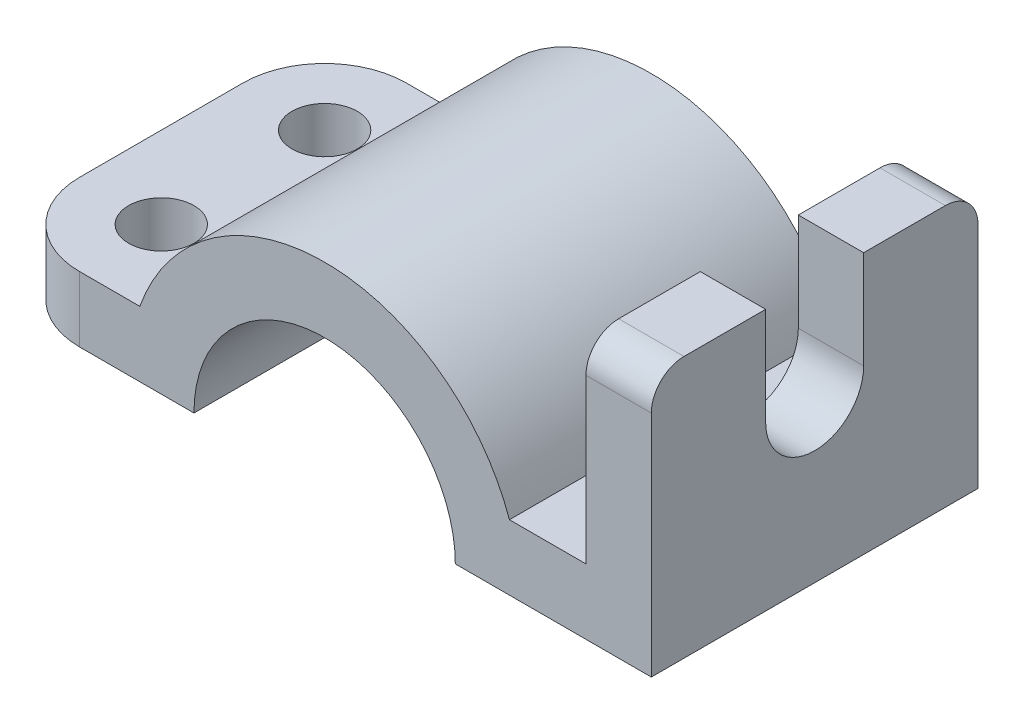
ISO-10303-21;
HEADER;
FILE_DESCRIPTION(('STEP AP214'),'2;1');
FILE_NAME('part.step','',(''),(''),'','','');
FILE_SCHEMA(('AUTOMOTIVE_DESIGN { 1 0 10303 214 1 1 1 1 }'));
ENDSEC;
DATA;
#1=APPLICATION_CONTEXT('core data for automotive mechanical design processes');
#2=APPLICATION_PROTOCOL_DEFINITION('international standard','automotive_design',2000,#1);
#3=PRODUCT_CONTEXT('',#1,'mechanical');
#4=PRODUCT('Part','Part','',(#3));
#5=PRODUCT_RELATED_PRODUCT_CATEGORY('part','',(#4));
#6=PRODUCT_DEFINITION_FORMATION('','',#4);
#7=PRODUCT_DEFINITION_CONTEXT('part definition',#1,'design');
#8=PRODUCT_DEFINITION('design','',#6,#7);
#9=PRODUCT_DEFINITION_SHAPE('','',#8);
#10=(LENGTH_UNIT() NAMED_UNIT(*) SI_UNIT(.MILLI.,.METRE.));
#11=(NAMED_UNIT(*) PLANE_ANGLE_UNIT() SI_UNIT($,.RADIAN.));
#12=(NAMED_UNIT(*) SI_UNIT($,.STERADIAN.) SOLID_ANGLE_UNIT());
#13=UNCERTAINTY_MEASURE_WITH_UNIT(LENGTH_MEASURE(1.E-05),#10,'distance_accuracy_value','');
#14=(GEOMETRIC_REPRESENTATION_CONTEXT(3) GLOBAL_UNCERTAINTY_ASSIGNED_CONTEXT((#13)) GLOBAL_UNIT_ASSIGNED_CONTEXT((#10,
#11,#12)) REPRESENTATION_CONTEXT('',''));
#15=CARTESIAN_POINT('',(0.,0.,0.));
#16=DIRECTION('',(0.,0.,1.));
#17=DIRECTION('',(1.,0.,0.));
#18=AXIS2_PLACEMENT_3D('',#15,#16,#17);
#19=CARTESIAN_POINT('',(0.,0.,50.));
#20=DIRECTION('',(0.,1.,0.));
#21=DIRECTION('',(0.,0.,1.));
#22=AXIS2_PLACEMENT_3D('',#19,#20,#21);
#23=PLANE('',#22);
#24=CARTESIAN_POINT('',(12.5,0.,37.5));
#25=DIRECTION('',(0.,1.,0.));
#26=DIRECTION('',(0.,0.,1.));
#27=AXIS2_PLACEMENT_3D('',#24,#25,#26);
#28=CIRCLE('',#27,5.00000000000001);
#29=CARTESIAN_POINT('',(12.5,0.,42.5));
#30=VERTEX_POINT('',#29);
#31=EDGE_CURVE('E331',#30,#30,#28,.T.);
#32=ORIENTED_EDGE('',*,*,#31,.T.);
#33=EDGE_LOOP('',(#32));
#34=FACE_BOUND('',#33,.T.);
#35=CARTESIAN_POINT('',(12.5,0.,12.5));
#36=DIRECTION('',(0.,1.,0.));
#37=DIRECTION('',(0.,0.,1.));
#38=AXIS2_PLACEMENT_3D('',#35,#36,#37);
#39=CIRCLE('',#38,5.);
#40=CARTESIAN_POINT('',(12.5,0.,17.5));
#41=VERTEX_POINT('',#40);
#42=EDGE_CURVE('E333',#41,#41,#39,.T.);
#43=ORIENTED_EDGE('',*,*,#42,.T.);
#44=EDGE_LOOP('',(#43));
#45=FACE_BOUND('',#44,.T.);
#46=DIRECTION('',(1.,0.,0.));
#47=VECTOR('',#46,1.);
#48=CARTESIAN_POINT('',(0.,0.,0.));
#49=LINE('',#48,#47);
#50=CARTESIAN_POINT('',(12.5,0.,0.));
#51=VERTEX_POINT('',#50);
#52=CARTESIAN_POINT('',(30.,0.,0.));
#53=VERTEX_POINT('',#52);
#54=EDGE_CURVE('E193',#51,#53,#49,.T.);
#55=ORIENTED_EDGE('',*,*,#54,.T.);
#56=DIRECTION('',(0.,0.,1.));
#57=VECTOR('',#56,1.);
#58=CARTESIAN_POINT('',(30.,0.,0.));
#59=LINE('',#58,#57);
#60=CARTESIAN_POINT('',(30.,0.,50.));
#61=VERTEX_POINT('',#60);
#62=EDGE_CURVE('E65',#53,#61,#59,.T.);
#63=ORIENTED_EDGE('',*,*,#62,.T.);
#64=DIRECTION('',(1.,0.,0.));
#65=VECTOR('',#64,1.);
#66=CARTESIAN_POINT('',(0.,0.,50.));
#67=LINE('',#66,#65);
#68=CARTESIAN_POINT('',(12.5,0.,50.));
#69=VERTEX_POINT('',#68);
#70=EDGE_CURVE('E294',#69,#61,#67,.T.);
#71=ORIENTED_EDGE('',*,*,#70,.F.);
#72=CARTESIAN_POINT('',(12.5,0.,37.5));
#73=DIRECTION('',(0.,1.,0.));
#74=DIRECTION('',(0.,0.,1.));
#75=AXIS2_PLACEMENT_3D('',#72,#73,#74);
#76=CIRCLE('',#75,12.5);
#77=CARTESIAN_POINT('',(0.,0.,37.5));
#78=VERTEX_POINT('',#77);
#79=EDGE_CURVE('E253',#69,#78,#76,.F.);
#80=ORIENTED_EDGE('',*,*,#79,.T.);
#81=DIRECTION('',(0.,0.,-1.));
#82=VECTOR('',#81,1.);
#83=CARTESIAN_POINT('',(0.,0.,50.));
#84=LINE('',#83,#82);
#85=CARTESIAN_POINT('',(0.,0.,12.5));
#86=VERTEX_POINT('',#85);
#87=EDGE_CURVE('E227',#78,#86,#84,.T.);
#88=ORIENTED_EDGE('',*,*,#87,.T.);
#89=CARTESIAN_POINT('',(12.5,0.,12.5));
#90=DIRECTION('',(0.,1.,0.));
#91=DIRECTION('',(0.,0.,1.));
#92=AXIS2_PLACEMENT_3D('',#89,#90,#91);
#93=CIRCLE('',#92,12.5);
#94=EDGE_CURVE('E247',#86,#51,#93,.F.);
#95=ORIENTED_EDGE('',*,*,#94,.T.);
#96=EDGE_LOOP('',(#55,#63,#71,#80,#88,#95));
#97=FACE_BOUND('',#96,.T.);
#98=ADVANCED_FACE('F50',(#34,#45,#97),#23,.F.);
#99=CARTESIAN_POINT('',(0.,10.,50.));
#100=DIRECTION('',(0.,-1.,0.));
#101=DIRECTION('',(0.,0.,-1.));
#102=AXIS2_PLACEMENT_3D('',#99,#100,#101);
#103=PLANE('',#102);
#104=DIRECTION('',(-1.,0.,0.));
#105=VECTOR('',#104,1.);
#106=CARTESIAN_POINT('',(0.,10.,0.));
#107=LINE('',#106,#105);
#108=CARTESIAN_POINT('',(90.,10.,0.));
#109=VERTEX_POINT('',#108);
#110=CARTESIAN_POINT('',(78.2842712474619,10.,0.));
#111=VERTEX_POINT('',#110);
#112=EDGE_CURVE('E209',#109,#111,#107,.T.);
#113=ORIENTED_EDGE('',*,*,#112,.T.);
#114=DIRECTION('',(0.,0.,1.));
#115=VECTOR('',#114,1.);
#116=CARTESIAN_POINT('',(78.2842712474619,10.,0.));
#117=LINE('',#116,#115);
#118=CARTESIAN_POINT('',(78.2842712474619,10.,50.));
#119=VERTEX_POINT('',#118);
#120=EDGE_CURVE('E314',#111,#119,#117,.T.);
#121=ORIENTED_EDGE('',*,*,#120,.T.);
#122=DIRECTION('',(-1.,0.,0.));
#123=VECTOR('',#122,1.);
#124=CARTESIAN_POINT('',(0.,10.,50.));
#125=LINE('',#124,#123);
#126=CARTESIAN_POINT('',(90.,10.,50.));
#127=VERTEX_POINT('',#126);
#128=EDGE_CURVE('E204',#127,#119,#125,.T.);
#129=ORIENTED_EDGE('',*,*,#128,.F.);
#130=DIRECTION('',(0.,0.,-1.));
#131=VECTOR('',#130,1.);
#132=CARTESIAN_POINT('',(90.,10.,50.));
#133=LINE('',#132,#131);
#134=EDGE_CURVE('E211',#127,#109,#133,.T.);
#135=ORIENTED_EDGE('',*,*,#134,.T.);
#136=EDGE_LOOP('',(#113,#121,#129,#135));
#137=FACE_BOUND('',#136,.T.);
#138=ADVANCED_FACE('F354',(#137),#103,.F.);
#139=CARTESIAN_POINT('',(0.,0.,50.));
#140=DIRECTION('',(1.,0.,0.));
#141=DIRECTION('',(0.,0.,-1.));
#142=AXIS2_PLACEMENT_3D('',#139,#140,#141);
#143=PLANE('',#142);
#144=DIRECTION('',(0.,1.,0.));
#145=VECTOR('',#144,1.);
#146=CARTESIAN_POINT('',(0.,-40.,37.5));
#147=LINE('',#146,#145);
#148=CARTESIAN_POINT('',(0.,10.,37.5));
#149=VERTEX_POINT('',#148);
#150=EDGE_CURVE('E257',#78,#149,#147,.T.);
#151=ORIENTED_EDGE('',*,*,#150,.T.);
#152=DIRECTION('',(0.,0.,-1.));
#153=VECTOR('',#152,1.);
#154=CARTESIAN_POINT('',(0.,10.,50.));
#155=LINE('',#154,#153);
#156=CARTESIAN_POINT('',(0.,10.,12.5));
#157=VERTEX_POINT('',#156);
#158=EDGE_CURVE('E212',#149,#157,#155,.T.);
#159=ORIENTED_EDGE('',*,*,#158,.T.);
#160=DIRECTION('',(0.,1.,0.));
#161=VECTOR('',#160,1.);
#162=CARTESIAN_POINT('',(0.,-40.,12.5));
#163=LINE('',#162,#161);
#164=EDGE_CURVE('E263',#86,#157,#163,.T.);
#165=ORIENTED_EDGE('',*,*,#164,.F.);
#166=ORIENTED_EDGE('',*,*,#87,.F.);
#167=EDGE_LOOP('',(#151,#159,#165,#166));
#168=FACE_BOUND('',#167,.T.);
#169=ADVANCED_FACE('F47',(#168),#143,.F.);
#170=CARTESIAN_POINT('',(70.,0.,50.));
#171=VERTEX_POINT('',#170);
#172=CARTESIAN_POINT('',(100.,0.,50.));
#173=VERTEX_POINT('',#172);
#174=EDGE_CURVE('E190',#171,#173,#67,.T.);
#175=ORIENTED_EDGE('',*,*,#174,.F.);
#176=DIRECTION('',(0.,0.,1.));
#177=VECTOR('',#176,1.);
#178=CARTESIAN_POINT('',(70.,0.,0.));
#179=LINE('',#178,#177);
#180=CARTESIAN_POINT('',(70.,0.,0.));
#181=VERTEX_POINT('',#180);
#182=EDGE_CURVE('E173',#181,#171,#179,.T.);
#183=ORIENTED_EDGE('',*,*,#182,.F.);
#184=CARTESIAN_POINT('',(100.,0.,0.));
#185=VERTEX_POINT('',#184);
#186=EDGE_CURVE('E184',#181,#185,#49,.T.);
#187=ORIENTED_EDGE('',*,*,#186,.T.);
#188=DIRECTION('',(0.,0.,-1.));
#189=VECTOR('',#188,1.);
#190=CARTESIAN_POINT('',(100.,0.,50.));
#191=LINE('',#190,#189);
#192=EDGE_CURVE('E225',#173,#185,#191,.T.);
#193=ORIENTED_EDGE('',*,*,#192,.F.);
#194=EDGE_LOOP('',(#175,#183,#187,#193));
#195=FACE_BOUND('',#194,.T.);
#196=ADVANCED_FACE('F182',(#195),#23,.F.);
#197=CARTESIAN_POINT('',(12.5,10.,37.5));
#198=DIRECTION('',(0.,1.,0.));
#199=DIRECTION('',(0.,0.,1.));
#200=AXIS2_PLACEMENT_3D('',#197,#198,#199);
#201=CIRCLE('',#200,5.00000000000001);
#202=CARTESIAN_POINT('',(12.5,10.,42.5));
#203=VERTEX_POINT('',#202);
#204=EDGE_CURVE('E339',#203,#203,#201,.T.);
#205=ORIENTED_EDGE('',*,*,#204,.F.);
#206=EDGE_LOOP('',(#205));
#207=FACE_BOUND('',#206,.T.);
#208=CARTESIAN_POINT('',(12.5,10.,12.5));
#209=DIRECTION('',(0.,1.,0.));
#210=DIRECTION('',(0.,0.,1.));
#211=AXIS2_PLACEMENT_3D('',#208,#209,#210);
#212=CIRCLE('',#211,5.);
#213=CARTESIAN_POINT('',(12.5,10.,17.5));
#214=VERTEX_POINT('',#213);
#215=EDGE_CURVE('E338',#214,#214,#212,.T.);
#216=ORIENTED_EDGE('',*,*,#215,.F.);
#217=EDGE_LOOP('',(#216));
#218=FACE_BOUND('',#217,.T.);
#219=CARTESIAN_POINT('',(21.7157287525381,10.,50.));
#220=VERTEX_POINT('',#219);
#221=CARTESIAN_POINT('',(12.5,10.,50.));
#222=VERTEX_POINT('',#221);
#223=EDGE_CURVE('E69',#220,#222,#125,.T.);
#224=ORIENTED_EDGE('',*,*,#223,.F.);
#225=DIRECTION('',(0.,0.,1.));
#226=VECTOR('',#225,1.);
#227=CARTESIAN_POINT('',(21.7157287525381,10.,0.));
#228=LINE('',#227,#226);
#229=CARTESIAN_POINT('',(21.7157287525381,10.,0.));
#230=VERTEX_POINT('',#229);
#231=EDGE_CURVE('E320',#230,#220,#228,.T.);
#232=ORIENTED_EDGE('',*,*,#231,.F.);
#233=CARTESIAN_POINT('',(12.5,10.,0.));
#234=VERTEX_POINT('',#233);
#235=EDGE_CURVE('E206',#230,#234,#107,.T.);
#236=ORIENTED_EDGE('',*,*,#235,.T.);
#237=CARTESIAN_POINT('',(12.5,10.,12.5));
#238=DIRECTION('',(0.,-1.,0.));
#239=DIRECTION('',(0.,0.,1.));
#240=AXIS2_PLACEMENT_3D('',#237,#238,#239);
#241=CIRCLE('',#240,12.5);
#242=EDGE_CURVE('E252',#157,#234,#241,.T.);
#243=ORIENTED_EDGE('',*,*,#242,.F.);
#244=ORIENTED_EDGE('',*,*,#158,.F.);
#245=CARTESIAN_POINT('',(12.5,10.,37.5));
#246=DIRECTION('',(0.,-1.,0.));
#247=DIRECTION('',(0.,0.,1.));
#248=AXIS2_PLACEMENT_3D('',#245,#246,#247);
#249=CIRCLE('',#248,12.5);
#250=EDGE_CURVE('E261',#222,#149,#249,.T.);
#251=ORIENTED_EDGE('',*,*,#250,.F.);
#252=EDGE_LOOP('',(#224,#232,#236,#243,#244,#251));
#253=FACE_BOUND('',#252,.T.);
#254=ADVANCED_FACE('F330',(#207,#218,#253),#103,.F.);
#255=CARTESIAN_POINT('',(100.,40.,50.));
#256=DIRECTION('',(0.,-1.,0.));
#257=DIRECTION('',(0.,0.,-1.));
#258=AXIS2_PLACEMENT_3D('',#255,#256,#257);
#259=PLANE('',#258);
#260=DIRECTION('',(0.,0.,-1.));
#261=VECTOR('',#260,1.);
#262=CARTESIAN_POINT('',(100.,40.,50.));
#263=LINE('',#262,#261);
#264=CARTESIAN_POINT('',(100.,40.,45.));
#265=VERTEX_POINT('',#264);
#266=CARTESIAN_POINT('',(100.,40.,32.5));
#267=VERTEX_POINT('',#266);
#268=EDGE_CURVE('E222',#265,#267,#263,.T.);
#269=ORIENTED_EDGE('',*,*,#268,.T.);
#270=DIRECTION('',(1.,0.,0.));
#271=VECTOR('',#270,1.);
#272=CARTESIAN_POINT('',(50.,40.,32.5));
#273=LINE('',#272,#271);
#274=CARTESIAN_POINT('',(90.,40.,32.5));
#275=VERTEX_POINT('',#274);
#276=EDGE_CURVE('E273',#275,#267,#273,.T.);
#277=ORIENTED_EDGE('',*,*,#276,.F.);
#278=DIRECTION('',(0.,0.,-1.));
#279=VECTOR('',#278,1.);
#280=CARTESIAN_POINT('',(90.,40.,50.));
#281=LINE('',#280,#279);
#282=CARTESIAN_POINT('',(90.,40.,45.));
#283=VERTEX_POINT('',#282);
#284=EDGE_CURVE('E217',#283,#275,#281,.T.);
#285=ORIENTED_EDGE('',*,*,#284,.F.);
#286=DIRECTION('',(1.,0.,0.));
#287=VECTOR('',#286,1.);
#288=CARTESIAN_POINT('',(50.,40.,45.));
#289=LINE('',#288,#287);
#290=EDGE_CURVE('E286',#283,#265,#289,.T.);
#291=ORIENTED_EDGE('',*,*,#290,.T.);
#292=EDGE_LOOP('',(#269,#277,#285,#291));
#293=FACE_BOUND('',#292,.T.);
#294=ADVANCED_FACE('F351',(#293),#259,.F.);
#295=CARTESIAN_POINT('',(100.,0.,50.));
#296=DIRECTION('',(-1.,0.,0.));
#297=DIRECTION('',(0.,0.,1.));
#298=AXIS2_PLACEMENT_3D('',#295,#296,#297);
#299=PLANE('',#298);
#300=CARTESIAN_POINT('',(100.,25.,25.));
#301=DIRECTION('',(1.,0.,0.));
#302=DIRECTION('',(0.,0.,-1.));
#303=AXIS2_PLACEMENT_3D('',#300,#301,#302);
#304=CIRCLE('',#303,7.5);
#305=CARTESIAN_POINT('',(100.,25.,32.5));
#306=VERTEX_POINT('',#305);
#307=CARTESIAN_POINT('',(100.,25.,17.5));
#308=VERTEX_POINT('',#307);
#309=EDGE_CURVE('E268',#306,#308,#304,.T.);
#310=ORIENTED_EDGE('',*,*,#309,.F.);
#311=DIRECTION('',(0.,-1.,0.));
#312=VECTOR('',#311,1.);
#313=CARTESIAN_POINT('',(100.,0.,32.5));
#314=LINE('',#313,#312);
#315=EDGE_CURVE('E259',#267,#306,#314,.T.);
#316=ORIENTED_EDGE('',*,*,#315,.F.);
#317=ORIENTED_EDGE('',*,*,#268,.F.);
#318=CARTESIAN_POINT('',(100.,35.,45.));
#319=DIRECTION('',(-1.,0.,0.));
#320=DIRECTION('',(0.,0.,-1.));
#321=AXIS2_PLACEMENT_3D('',#318,#319,#320);
#322=CIRCLE('',#321,5.);
#323=CARTESIAN_POINT('',(100.,35.,50.));
#324=VERTEX_POINT('',#323);
#325=EDGE_CURVE('E283',#324,#265,#322,.T.);
#326=ORIENTED_EDGE('',*,*,#325,.F.);
#327=DIRECTION('',(0.,1.,0.));
#328=VECTOR('',#327,1.);
#329=CARTESIAN_POINT('',(100.,0.,50.));
#330=LINE('',#329,#328);
#331=EDGE_CURVE('E296',#173,#324,#330,.T.);
#332=ORIENTED_EDGE('',*,*,#331,.F.);
#333=ORIENTED_EDGE('',*,*,#192,.T.);
#334=DIRECTION('',(0.,1.,0.));
#335=VECTOR('',#334,1.);
#336=CARTESIAN_POINT('',(100.,0.,0.));
#337=LINE('',#336,#335);
#338=CARTESIAN_POINT('',(100.,35.,0.));
#339=VERTEX_POINT('',#338);
#340=EDGE_CURVE('E191',#185,#339,#337,.T.);
#341=ORIENTED_EDGE('',*,*,#340,.T.);
#342=CARTESIAN_POINT('',(100.,35.,5.));
#343=DIRECTION('',(-1.,0.,0.));
#344=DIRECTION('',(0.,0.,-1.));
#345=AXIS2_PLACEMENT_3D('',#342,#343,#344);
#346=CIRCLE('',#345,5.);
#347=CARTESIAN_POINT('',(100.,40.,5.));
#348=VERTEX_POINT('',#347);
#349=EDGE_CURVE('E280',#348,#339,#346,.T.);
#350=ORIENTED_EDGE('',*,*,#349,.F.);
#351=CARTESIAN_POINT('',(100.,40.,17.5));
#352=VERTEX_POINT('',#351);
#353=EDGE_CURVE('E221',#352,#348,#263,.T.);
#354=ORIENTED_EDGE('',*,*,#353,.F.);
#355=DIRECTION('',(0.,1.,0.));
#356=VECTOR('',#355,1.);
#357=CARTESIAN_POINT('',(100.,0.,17.5));
#358=LINE('',#357,#356);
#359=EDGE_CURVE('E275',#308,#352,#358,.T.);
#360=ORIENTED_EDGE('',*,*,#359,.F.);
#361=EDGE_LOOP('',(#310,#316,#317,#326,#332,#333,#341,#350,#354,#360));
#362=FACE_BOUND('',#361,.T.);
#363=ADVANCED_FACE('F494',(#362),#299,.F.);
#364=CARTESIAN_POINT('',(90.,40.,17.5));
#365=VERTEX_POINT('',#364);
#366=CARTESIAN_POINT('',(90.,40.,5.));
#367=VERTEX_POINT('',#366);
#368=EDGE_CURVE('E220',#365,#367,#281,.T.);
#369=ORIENTED_EDGE('',*,*,#368,.F.);
#370=DIRECTION('',(1.,0.,0.));
#371=VECTOR('',#370,1.);
#372=CARTESIAN_POINT('',(50.,40.,17.5));
#373=LINE('',#372,#371);
#374=EDGE_CURVE('E279',#365,#352,#373,.T.);
#375=ORIENTED_EDGE('',*,*,#374,.T.);
#376=ORIENTED_EDGE('',*,*,#353,.T.);
#377=DIRECTION('',(1.,0.,0.));
#378=VECTOR('',#377,1.);
#379=CARTESIAN_POINT('',(50.,40.,5.));
#380=LINE('',#379,#378);
#381=EDGE_CURVE('E287',#367,#348,#380,.T.);
#382=ORIENTED_EDGE('',*,*,#381,.F.);
#383=EDGE_LOOP('',(#369,#375,#376,#382));
#384=FACE_BOUND('',#383,.T.);
#385=ADVANCED_FACE('F483',(#384),#259,.F.);
#386=CARTESIAN_POINT('',(90.,10.,50.));
#387=DIRECTION('',(1.,0.,0.));
#388=DIRECTION('',(0.,0.,-1.));
#389=AXIS2_PLACEMENT_3D('',#386,#387,#388);
#390=PLANE('',#389);
#391=ORIENTED_EDGE('',*,*,#284,.T.);
#392=DIRECTION('',(0.,-1.,0.));
#393=VECTOR('',#392,1.);
#394=CARTESIAN_POINT('',(90.,10.,32.5));
#395=LINE('',#394,#393);
#396=CARTESIAN_POINT('',(90.,25.,32.5));
#397=VERTEX_POINT('',#396);
#398=EDGE_CURVE('E241',#275,#397,#395,.T.);
#399=ORIENTED_EDGE('',*,*,#398,.T.);
#400=CARTESIAN_POINT('',(90.,25.,25.));
#401=DIRECTION('',(1.,0.,0.));
#402=DIRECTION('',(0.,0.,-1.));
#403=AXIS2_PLACEMENT_3D('',#400,#401,#402);
#404=CIRCLE('',#403,7.5);
#405=CARTESIAN_POINT('',(90.,25.,17.5));
#406=VERTEX_POINT('',#405);
#407=EDGE_CURVE('E232',#397,#406,#404,.T.);
#408=ORIENTED_EDGE('',*,*,#407,.T.);
#409=DIRECTION('',(0.,1.,0.));
#410=VECTOR('',#409,1.);
#411=CARTESIAN_POINT('',(90.,10.,17.5));
#412=LINE('',#411,#410);
#413=EDGE_CURVE('E238',#406,#365,#412,.T.);
#414=ORIENTED_EDGE('',*,*,#413,.T.);
#415=ORIENTED_EDGE('',*,*,#368,.T.);
#416=CARTESIAN_POINT('',(90.,35.,5.));
#417=DIRECTION('',(1.,0.,0.));
#418=DIRECTION('',(0.,0.,-1.));
#419=AXIS2_PLACEMENT_3D('',#416,#417,#418);
#420=CIRCLE('',#419,5.);
#421=CARTESIAN_POINT('',(90.,35.,0.));
#422=VERTEX_POINT('',#421);
#423=EDGE_CURVE('E198',#367,#422,#420,.F.);
#424=ORIENTED_EDGE('',*,*,#423,.T.);
#425=DIRECTION('',(0.,-1.,0.));
#426=VECTOR('',#425,1.);
#427=CARTESIAN_POINT('',(90.,10.,0.));
#428=LINE('',#427,#426);
#429=EDGE_CURVE('E207',#422,#109,#428,.T.);
#430=ORIENTED_EDGE('',*,*,#429,.T.);
#431=ORIENTED_EDGE('',*,*,#134,.F.);
#432=DIRECTION('',(0.,-1.,0.));
#433=VECTOR('',#432,1.);
#434=CARTESIAN_POINT('',(90.,10.,50.));
#435=LINE('',#434,#433);
#436=CARTESIAN_POINT('',(90.,35.,50.));
#437=VERTEX_POINT('',#436);
#438=EDGE_CURVE('E297',#437,#127,#435,.T.);
#439=ORIENTED_EDGE('',*,*,#438,.F.);
#440=CARTESIAN_POINT('',(90.,35.,45.));
#441=DIRECTION('',(1.,0.,0.));
#442=DIRECTION('',(0.,0.,-1.));
#443=AXIS2_PLACEMENT_3D('',#440,#441,#442);
#444=CIRCLE('',#443,5.);
#445=EDGE_CURVE('E196',#437,#283,#444,.F.);
#446=ORIENTED_EDGE('',*,*,#445,.T.);
#447=EDGE_LOOP('',(#391,#399,#408,#414,#415,#424,#430,#431,#439,#446));
#448=FACE_BOUND('',#447,.T.);
#449=ADVANCED_FACE('F479',(#448),#390,.F.);
#450=CARTESIAN_POINT('',(0.,0.,50.));
#451=DIRECTION('',(0.,0.,-1.));
#452=DIRECTION('',(-1.,0.,0.));
#453=AXIS2_PLACEMENT_3D('',#450,#451,#452);
#454=PLANE('',#453);
#455=ORIENTED_EDGE('',*,*,#70,.T.);
#456=CARTESIAN_POINT('',(50.,0.,50.));
#457=DIRECTION('',(0.,0.,1.));
#458=DIRECTION('',(1.,0.,0.));
#459=AXIS2_PLACEMENT_3D('',#456,#457,#458);
#460=CIRCLE('',#459,20.);
#461=EDGE_CURVE('E177',#171,#61,#460,.T.);
#462=ORIENTED_EDGE('',*,*,#461,.F.);
#463=ORIENTED_EDGE('',*,*,#174,.T.);
#464=ORIENTED_EDGE('',*,*,#331,.T.);
#465=DIRECTION('',(1.,0.,0.));
#466=VECTOR('',#465,1.);
#467=CARTESIAN_POINT('',(50.,35.,50.));
#468=LINE('',#467,#466);
#469=EDGE_CURVE('E235',#324,#437,#468,.F.);
#470=ORIENTED_EDGE('',*,*,#469,.T.);
#471=ORIENTED_EDGE('',*,*,#438,.T.);
#472=ORIENTED_EDGE('',*,*,#128,.T.);
#473=CARTESIAN_POINT('',(50.,0.,50.));
#474=DIRECTION('',(0.,0.,1.));
#475=DIRECTION('',(1.,0.,0.));
#476=AXIS2_PLACEMENT_3D('',#473,#474,#475);
#477=CIRCLE('',#476,30.);
#478=EDGE_CURVE('E189',#119,#220,#477,.T.);
#479=ORIENTED_EDGE('',*,*,#478,.T.);
#480=ORIENTED_EDGE('',*,*,#223,.T.);
#481=DIRECTION('',(0.,1.,0.));
#482=VECTOR('',#481,1.);
#483=CARTESIAN_POINT('',(12.5,-40.,50.));
#484=LINE('',#483,#482);
#485=EDGE_CURVE('E11',#222,#69,#484,.F.);
#486=ORIENTED_EDGE('',*,*,#485,.T.);
#487=EDGE_LOOP('',(#455,#462,#463,#464,#470,#471,#472,#479,#480,#486));
#488=FACE_BOUND('',#487,.T.);
#489=ADVANCED_FACE('F307',(#488),#454,.F.);
#490=CARTESIAN_POINT('',(0.,0.,0.));
#491=DIRECTION('',(0.,0.,-1.));
#492=DIRECTION('',(-1.,0.,0.));
#493=AXIS2_PLACEMENT_3D('',#490,#491,#492);
#494=PLANE('',#493);
#495=CARTESIAN_POINT('',(50.,0.,0.));
#496=DIRECTION('',(0.,0.,1.));
#497=DIRECTION('',(1.,0.,0.));
#498=AXIS2_PLACEMENT_3D('',#495,#496,#497);
#499=CIRCLE('',#498,20.);
#500=EDGE_CURVE('E167',#181,#53,#499,.T.);
#501=ORIENTED_EDGE('',*,*,#500,.T.);
#502=ORIENTED_EDGE('',*,*,#54,.F.);
#503=DIRECTION('',(0.,1.,0.));
#504=VECTOR('',#503,1.);
#505=CARTESIAN_POINT('',(12.5,-40.,0.));
#506=LINE('',#505,#504);
#507=EDGE_CURVE('E54',#234,#51,#506,.F.);
#508=ORIENTED_EDGE('',*,*,#507,.F.);
#509=ORIENTED_EDGE('',*,*,#235,.F.);
#510=CARTESIAN_POINT('',(50.,0.,0.));
#511=DIRECTION('',(0.,0.,1.));
#512=DIRECTION('',(1.,0.,0.));
#513=AXIS2_PLACEMENT_3D('',#510,#511,#512);
#514=CIRCLE('',#513,30.);
#515=EDGE_CURVE('E319',#111,#230,#514,.T.);
#516=ORIENTED_EDGE('',*,*,#515,.F.);
#517=ORIENTED_EDGE('',*,*,#112,.F.);
#518=ORIENTED_EDGE('',*,*,#429,.F.);
#519=DIRECTION('',(1.,0.,0.));
#520=VECTOR('',#519,1.);
#521=CARTESIAN_POINT('',(50.,35.,0.));
#522=LINE('',#521,#520);
#523=EDGE_CURVE('E229',#339,#422,#522,.F.);
#524=ORIENTED_EDGE('',*,*,#523,.F.);
#525=ORIENTED_EDGE('',*,*,#340,.F.);
#526=ORIENTED_EDGE('',*,*,#186,.F.);
#527=EDGE_LOOP('',(#501,#502,#508,#509,#516,#517,#518,#524,#525,#526));
#528=FACE_BOUND('',#527,.T.);
#529=ADVANCED_FACE('F192',(#528),#494,.T.);
#530=CARTESIAN_POINT('',(50.,35.,5.));
#531=DIRECTION('',(1.,0.,0.));
#532=DIRECTION('',(0.,0.,-1.));
#533=AXIS2_PLACEMENT_3D('',#530,#531,#532);
#534=CYLINDRICAL_SURFACE('',#533,5.);
#535=ORIENTED_EDGE('',*,*,#381,.T.);
#536=ORIENTED_EDGE('',*,*,#349,.T.);
#537=ORIENTED_EDGE('',*,*,#523,.T.);
#538=ORIENTED_EDGE('',*,*,#423,.F.);
#539=EDGE_LOOP('',(#535,#536,#537,#538));
#540=FACE_BOUND('',#539,.T.);
#541=ADVANCED_FACE('F513',(#540),#534,.T.);
#542=CARTESIAN_POINT('',(50.,35.,45.));
#543=DIRECTION('',(1.,0.,0.));
#544=DIRECTION('',(0.,0.,-1.));
#545=AXIS2_PLACEMENT_3D('',#542,#543,#544);
#546=CYLINDRICAL_SURFACE('',#545,5.);
#547=ORIENTED_EDGE('',*,*,#469,.F.);
#548=ORIENTED_EDGE('',*,*,#325,.T.);
#549=ORIENTED_EDGE('',*,*,#290,.F.);
#550=ORIENTED_EDGE('',*,*,#445,.F.);
#551=EDGE_LOOP('',(#547,#548,#549,#550));
#552=FACE_BOUND('',#551,.T.);
#553=ADVANCED_FACE('F469',(#552),#546,.T.);
#554=CARTESIAN_POINT('',(50.,0.,32.5));
#555=DIRECTION('',(0.,0.,1.));
#556=DIRECTION('',(1.,0.,0.));
#557=AXIS2_PLACEMENT_3D('',#554,#555,#556);
#558=PLANE('',#557);
#559=ORIENTED_EDGE('',*,*,#276,.T.);
#560=ORIENTED_EDGE('',*,*,#315,.T.);
#561=DIRECTION('',(1.,0.,0.));
#562=VECTOR('',#561,1.);
#563=CARTESIAN_POINT('',(50.,25.,32.5));
#564=LINE('',#563,#562);
#565=EDGE_CURVE('E274',#397,#306,#564,.T.);
#566=ORIENTED_EDGE('',*,*,#565,.F.);
#567=ORIENTED_EDGE('',*,*,#398,.F.);
#568=EDGE_LOOP('',(#559,#560,#566,#567));
#569=FACE_BOUND('',#568,.T.);
#570=ADVANCED_FACE('F459',(#569),#558,.F.);
#571=CARTESIAN_POINT('',(50.,0.,17.5));
#572=DIRECTION('',(0.,0.,-1.));
#573=DIRECTION('',(-1.,0.,0.));
#574=AXIS2_PLACEMENT_3D('',#571,#572,#573);
#575=PLANE('',#574);
#576=DIRECTION('',(1.,0.,0.));
#577=VECTOR('',#576,1.);
#578=CARTESIAN_POINT('',(50.,25.,17.5));
#579=LINE('',#578,#577);
#580=EDGE_CURVE('E281',#406,#308,#579,.T.);
#581=ORIENTED_EDGE('',*,*,#580,.T.);
#582=ORIENTED_EDGE('',*,*,#359,.T.);
#583=ORIENTED_EDGE('',*,*,#374,.F.);
#584=ORIENTED_EDGE('',*,*,#413,.F.);
#585=EDGE_LOOP('',(#581,#582,#583,#584));
#586=FACE_BOUND('',#585,.T.);
#587=ADVANCED_FACE('F454',(#586),#575,.F.);
#588=CARTESIAN_POINT('',(50.,25.,25.));
#589=DIRECTION('',(1.,0.,0.));
#590=DIRECTION('',(0.,0.,-1.));
#591=AXIS2_PLACEMENT_3D('',#588,#589,#590);
#592=CYLINDRICAL_SURFACE('',#591,7.5);
#593=ORIENTED_EDGE('',*,*,#565,.T.);
#594=ORIENTED_EDGE('',*,*,#309,.T.);
#595=ORIENTED_EDGE('',*,*,#580,.F.);
#596=ORIENTED_EDGE('',*,*,#407,.F.);
#597=EDGE_LOOP('',(#593,#594,#595,#596));
#598=FACE_BOUND('',#597,.T.);
#599=ADVANCED_FACE('F384',(#598),#592,.F.);
#600=CARTESIAN_POINT('',(12.5,-40.,12.5));
#601=DIRECTION('',(0.,1.,0.));
#602=DIRECTION('',(0.,0.,1.));
#603=AXIS2_PLACEMENT_3D('',#600,#601,#602);
#604=CYLINDRICAL_SURFACE('',#603,12.5);
#605=ORIENTED_EDGE('',*,*,#164,.T.);
#606=ORIENTED_EDGE('',*,*,#242,.T.);
#607=ORIENTED_EDGE('',*,*,#507,.T.);
#608=ORIENTED_EDGE('',*,*,#94,.F.);
#609=EDGE_LOOP('',(#605,#606,#607,#608));
#610=FACE_BOUND('',#609,.T.);
#611=ADVANCED_FACE('F250',(#610),#604,.T.);
#612=CARTESIAN_POINT('',(12.5,-40.,37.5));
#613=DIRECTION('',(0.,1.,0.));
#614=DIRECTION('',(0.,0.,1.));
#615=AXIS2_PLACEMENT_3D('',#612,#613,#614);
#616=CYLINDRICAL_SURFACE('',#615,12.5);
#617=ORIENTED_EDGE('',*,*,#485,.F.);
#618=ORIENTED_EDGE('',*,*,#250,.T.);
#619=ORIENTED_EDGE('',*,*,#150,.F.);
#620=ORIENTED_EDGE('',*,*,#79,.F.);
#621=EDGE_LOOP('',(#617,#618,#619,#620));
#622=FACE_BOUND('',#621,.T.);
#623=ADVANCED_FACE('F328',(#622),#616,.T.);
#624=CARTESIAN_POINT('',(50.,0.,0.));
#625=DIRECTION('',(0.,0.,1.));
#626=DIRECTION('',(1.,0.,0.));
#627=AXIS2_PLACEMENT_3D('',#624,#625,#626);
#628=CYLINDRICAL_SURFACE('',#627,30.);
#629=ORIENTED_EDGE('',*,*,#478,.F.);
#630=ORIENTED_EDGE('',*,*,#120,.F.);
#631=ORIENTED_EDGE('',*,*,#515,.T.);
#632=ORIENTED_EDGE('',*,*,#231,.T.);
#633=EDGE_LOOP('',(#629,#630,#631,#632));
#634=FACE_BOUND('',#633,.T.);
#635=ADVANCED_FACE('F312',(#634),#628,.T.);
#636=CARTESIAN_POINT('',(50.,0.,0.));
#637=DIRECTION('',(0.,0.,1.));
#638=DIRECTION('',(1.,0.,0.));
#639=AXIS2_PLACEMENT_3D('',#636,#637,#638);
#640=CYLINDRICAL_SURFACE('',#639,20.);
#641=ORIENTED_EDGE('',*,*,#461,.T.);
#642=ORIENTED_EDGE('',*,*,#62,.F.);
#643=ORIENTED_EDGE('',*,*,#500,.F.);
#644=ORIENTED_EDGE('',*,*,#182,.T.);
#645=EDGE_LOOP('',(#641,#642,#643,#644));
#646=FACE_BOUND('',#645,.T.);
#647=ADVANCED_FACE('F175',(#646),#640,.F.);
#648=CARTESIAN_POINT('',(12.5,-40.,12.5));
#649=DIRECTION('',(0.,1.,0.));
#650=DIRECTION('',(0.,0.,1.));
#651=AXIS2_PLACEMENT_3D('',#648,#649,#650);
#652=CYLINDRICAL_SURFACE('',#651,5.);
#653=ORIENTED_EDGE('',*,*,#215,.T.);
#654=EDGE_LOOP('',(#653));
#655=FACE_BOUND('',#654,.T.);
#656=ORIENTED_EDGE('',*,*,#42,.F.);
#657=EDGE_LOOP('',(#656));
#658=FACE_BOUND('',#657,.T.);
#659=ADVANCED_FACE('F358',(#655,#658),#652,.F.);
#660=CARTESIAN_POINT('',(12.5,-40.,37.5));
#661=DIRECTION('',(0.,1.,0.));
#662=DIRECTION('',(0.,0.,1.));
#663=AXIS2_PLACEMENT_3D('',#660,#661,#662);
#664=CYLINDRICAL_SURFACE('',#663,5.00000000000001);
#665=ORIENTED_EDGE('',*,*,#204,.T.);
#666=EDGE_LOOP('',(#665));
#667=FACE_BOUND('',#666,.T.);
#668=ORIENTED_EDGE('',*,*,#31,.F.);
#669=EDGE_LOOP('',(#668));
#670=FACE_BOUND('',#669,.T.);
#671=ADVANCED_FACE('F346',(#667,#670),#664,.F.);
#672=CLOSED_SHELL('',(#98,#138,#169,#196,#254,#294,#363,#385,#449,#489,#529,#541,#553,#570,#587,
#599,#611,#623,#635,#647,#659,#671));
#673=MANIFOLD_SOLID_BREP('B2',#672);
#674=ADVANCED_BREP_SHAPE_REPRESENTATION('',(#18,#673),#14);
#675=SHAPE_DEFINITION_REPRESENTATION(#9,#674);
ENDSEC;
END-ISO-10303-21;
